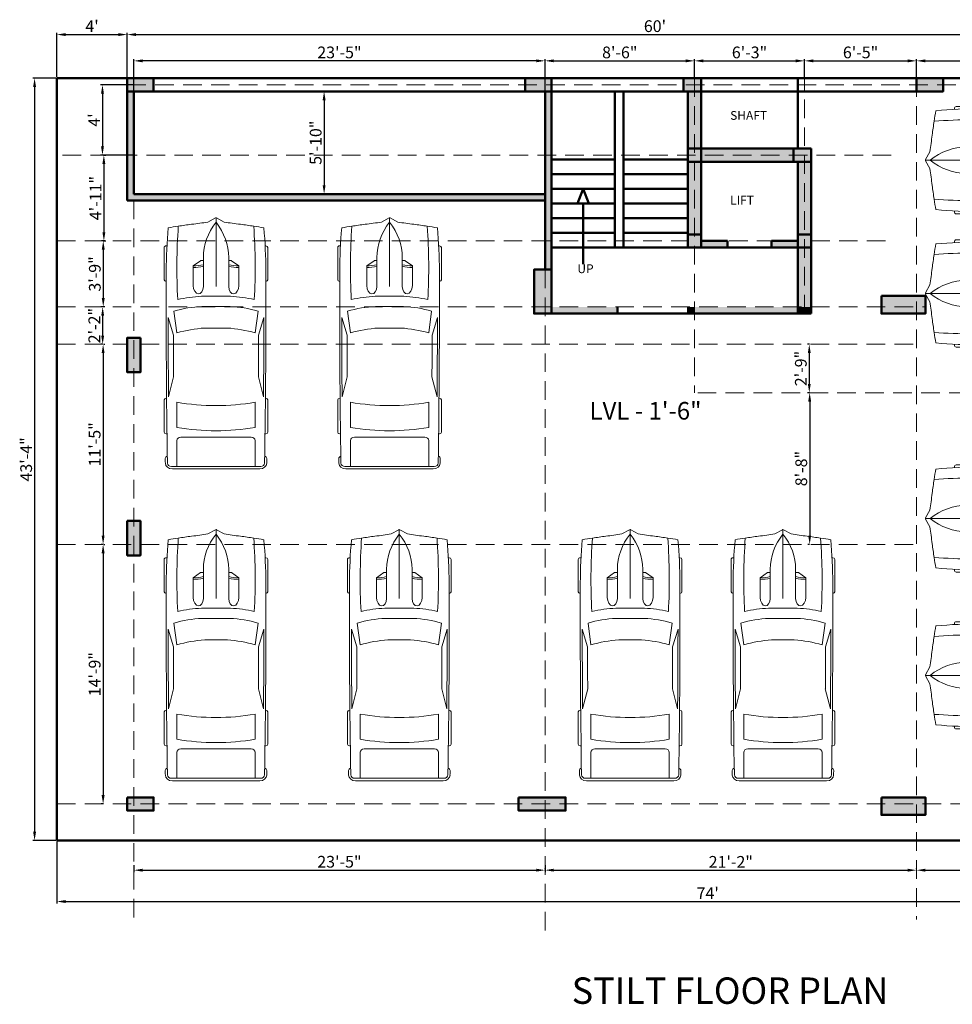
# Model space of a CAD drawing. Units: millimetres. Extents: x 1706 to 5913, y 156 to 1716.
# Tile 6 of 26: x 1714 to 2350, y 1031 to 1702. Entities that reach past the tile are written whole.
import ezdxf

# ---------------------------------------------------------------- set-up
doc = ezdxf.new("R2010")
doc.units = ezdxf.units.MM
doc.linetypes.add('DASHED', pattern=[19.05, 12.7, -6.35])
for name, color, linetype, lineweight in [('A-ANNO-DIMS', 2, 'Continuous', 18), ('A-ANNO-SYMB', 3, 'Continuous', 18), ('A-ANNO-TEXT', 7, 'Continuous', 18), ('A-AREA-IDEN', 3, 'Continuous', 18), ('A-COLS', 20, 'Continuous', 50), ('A-EQPM', 8, 'Continuous', 18), ('A-FLOR-OVHD', 9, 'DASHED', 18), ('A-WALL', 7, 'Continuous', 50), ('A-WALL-PATT', 252, 'Continuous', 13)]:
    doc.layers.add(name, color=color, linetype=linetype, lineweight=lineweight)
doc.styles.get("Standard").update_dxf_attribs({"font": 'arial.ttf'})
doc.dimstyles.new('ISO-25', dxfattribs={"dimtxt": 8, "dimasz": 6, "dimexe": 1.25, "dimexo": 0.625, "dimtad": 1, "dimdec": 0, "dimlunit": 3, "dimtxsty": 'Standard', "dimcen": 2.5, "dimadec": 0, "dimazin": 0, "dimtfac": 1, "dimtdec": 0, "dimtmove": 0, "dimatfit": 3, "dimfxl": 1, "dimarcsym": 0})

# ---------------------------------------------------------------- blocks, each defined once
blk = doc.blocks.new('*D81')
at = {"layer": 'A-ANNO-DIMS', "color": 0, "lineweight": -2, "transparency": 16777216}
for p, q in [((1771.16, 1609.78), (1772.72, 1609.78)), ((1771.47, 1603.78), (1771.47, 1557.28)), ((1771.16, 1551.28), (1772.72, 1551.28))]:
    blk.add_line(p, q, dxfattribs=at)
at = {"layer": 'A-ANNO-DIMS', "color": 0, "transparency": 16777216}
for points in [[(1770.47, 1603.78), (1772.47, 1603.78), (1771.47, 1609.78)], [(1770.47, 1557.28), (1772.47, 1557.28), (1771.47, 1551.28)]]:
    blk.add_solid(points, dxfattribs=at)
at = {"layer": 'Defpoints', "color": 0, "transparency": 16777216}
for p in [(1770.53, 1609.78), (1770.53, 1551.28), (1771.47, 1551.28)]:
    blk.add_point(p, dxfattribs=at)
at = {"layer": 'A-ANNO-DIMS', "color": 0, "transparency": 16777216, "insert": (1766.83, 1580.53), "char_height": 8, "attachment_point": 5, "rotation": 90}
blk.add_mtext('4\'-11"', dxfattribs=at)
blk = doc.blocks.new('*D82')
at = {"layer": 'A-ANNO-DIMS', "color": 0, "lineweight": -2, "transparency": 16777216}
for p, q in [((1772.1, 1551.28), (1769.8, 1551.28)), ((1771.05, 1545.28), (1771.05, 1512.28)), ((1772.1, 1506.28), (1769.8, 1506.28))]:
    blk.add_line(p, q, dxfattribs=at)
at = {"layer": 'A-ANNO-DIMS', "color": 0, "transparency": 16777216}
for points in [[(1770.05, 1545.28), (1772.05, 1545.28), (1771.05, 1551.28)], [(1770.05, 1512.28), (1772.05, 1512.28), (1771.05, 1506.28)]]:
    blk.add_solid(points, dxfattribs=at)
at = {"layer": 'Defpoints', "color": 0, "transparency": 16777216}
for p in [(1772.72, 1551.28), (1771.05, 1506.28), (1772.72, 1506.28)]:
    blk.add_point(p, dxfattribs=at)
at = {"layer": 'A-ANNO-DIMS', "color": 0, "transparency": 16777216, "insert": (1766.34, 1528.78), "char_height": 8, "attachment_point": 5, "rotation": 90}
blk.add_mtext('3\'-9"', dxfattribs=at)
blk = doc.blocks.new('*U10')
for p, q in [((21.1, 37.41), (21.1, 36.83)), ((46.55, 38.89), (22.35, 38.89)), ((47.8, 37.39), (47.8, 37.41)), ((87.99, 31.87), (74.76, 35.92)), ((135.45, 37.07), (135.45, 37.41)), ((136.7, 38.89), (160.9, 38.89)), ((162.15, 37.41), (162.15, 36.77)), ((70.03, 31.54), (86.41, 29.35)), ((134.31, 35.6), (119.29, 31.78)), ((138.42, 29.35), (157.25, 29.35)), ((186.47, 29.35), (167.01, 29.35)), ((186.47, -33.5), (186.47, 33.5)), ((188.4, -32.76), (188.4, 32.76)), ((164.52, 26.39), (164.52, -26.39)), ((32.27, 11.63), (36.13, 17.17)), ((36.13, 17.17), (50.94, 17.17)), ((29.77, 9.51), (51.68, 9.51)), ((32.12, 9.51), (32.12, 11.15)), ((58.92, -10.77), (58.92, 10.77)), ((66.55, -10.53), (66.55, 10.53)), ((82.74, 8.5), (82.74, -8.5)), ((186.47, -10.53), (186.47, 10.53)), ((3.27, 6.13), (0.1, 0.41)), ((0, 0), (51.68, 0)), ((0.1, -0.41), (3.27, -6.13)), ((29.77, -9.51), (51.68, -9.51)), ((32.12, -9.51), (32.12, -11.15)), ((32.27, -11.63), (36.13, -17.17)), ((36.13, -17.17), (50.94, -17.17)), ((86.41, -29.35), (70.03, -31.54)), ((87.99, -31.87), (74.76, -35.92)), ((134.31, -35.6), (119.29, -31.78)), ((157.25, -29.35), (138.42, -29.35)), ((167.01, -29.35), (186.47, -29.35)), ((21.1, -37.41), (21.1, -36.83)), ((46.55, -38.89), (22.35, -38.89)), ((47.8, -37.39), (47.8, -37.41)), ((135.45, -37.07), (135.45, -37.41)), ((136.7, -38.89), (160.9, -38.89)), ((162.15, -37.41), (162.15, -36.77))]:
    blk.add_line(p, q)
for centre, major_axis, ratio, start_param, end_param in [((266.03, -27.52), (0, 313.31), 0.842304, 1.367076, 1.39176), ((41.19, -490.86), (0, 528.23), 0.842304, 0.00281, 0.075598), ((22.35, 37.41), (0, -1.48), 0.842304, 3.141593, 4.712389), ((64.48, -10555.62), (0, 10593.03), 0.842304, -0.013397, 0.002797), ((46.55, 37.41), (0, 1.48), 0.842304, -1.570796, 0), ((64.48, -10555.62), (0, -10591.55), 0.842304, 3.133765, 3.140441), ((136.7, 37.41), (0, -1.48), 0.842304, 3.141593, 4.712389), ((160.9, 37.41), (0, 1.48), 0.842304, -1.570796, 0), ((180.63, 35.84), (0, 2.22), 0.842304, -0.013017, 1.249894), ((64.48, -10556.36), (0, 10595.31), 0.842304, -0.013397, -0.013017), ((183.98, 33.5), (0, -2.96), 0.842304, 1.570796, 3.128196), ((183.98, 32.76), (0, -5.25), 0.842304, 1.570796, 3.128196), ((37.47, -593.96), (0, -623.33), 0.842304, 3.096046, 3.200911), ((134.4, 5.39), (0, -89.78), 0.842304, 4.449482, 4.652344), ((135.29, 5.39), (0, 81.77), 0.842304, 1.245306, 1.50788), ((149.6, 2.8), (0, -79.58), 0.842304, 4.372215, 4.640744), ((95.79, -3666.35), (0, -3698.24), 0.842304, 3.134049, 3.144098), ((17.08, 0), (0, 147.02), 0.842304, 4.511394, 4.913384), ((35.91, 0), (0, 147.02), 0.842304, 4.511394, 4.913384), ((167.01, 26.39), (0, 2.96), 0.842304, 0, 1.570796), ((259.18, -27.52), (0, -305.3), 0.842304, 4.528606, 4.561838), ((-204.49, 52.4), (0, -250.96), 0.842304, 1.385369, 1.434372), ((13.04, 17.01), (0, 27.42), 0.842304, 4.435146, 4.718221), ((14.2, 17.01), (0, 27.42), 0.842304, 4.435146, 4.718221), ((50.79, 13.34), (6.34, -0.36), 0.603834, -1.395552, 1.581315), ((29.77, -46.66), (0, 56.17), 0.842304, 0, 0.590319), ((32.75, 11.15), (0, 0.74), 0.842304, 0.879714, 1.570796), ((0.62, 0), (0, -0.74), 0.842304, 4.131459, 5.293319), ((-204.49, -52.4), (0, 250.96), 0.842304, -1.434372, -1.385369), ((29.77, 46.66), (0, 56.17), 0.842304, 2.551274, 3.141593), ((32.75, -11.15), (0, -0.74), 0.842304, 4.712389, 5.403472), ((13.04, -17.01), (0, -27.42), 0.842304, 1.564964, 1.848039), ((14.2, -17.01), (0, -27.42), 0.842304, 1.564964, 1.848039), ((134.4, -5.39), (0, -89.78), 0.842304, -1.510751, -1.307889), ((135.29, -5.39), (0, -81.77), 0.842304, -1.50788, -1.245306), ((149.6, -2.8), (0, -79.58), 0.842304, -1.499151, -1.230623), ((259.18, 27.52), (0, 305.3), 0.842304, 1.721348, 1.754579), ((266.03, 27.52), (0, 313.31), 0.842304, 1.749832, 1.774517), ((37.47, 593.96), (0, -623.33), 0.842304, -0.059319, 0.045547), ((167.01, -26.39), (0, -2.96), 0.842304, 4.712389, 6.283185), ((64.48, 10555.62), (0, -10591.55), 0.842304, 0.001152, 0.007828), ((95.79, 3666.35), (0, -3698.24), 0.842304, -0.002505, 0.007544), ((183.98, -33.5), (0, 2.96), 0.842304, 3.15499, 4.712389), ((183.98, -32.76), (0, -5.25), 0.842304, 0.013397, 1.570796), ((41.19, 490.86), (0, -528.23), 0.842304, -0.075598, -0.00281), ((22.35, -37.41), (0, 1.48), 0.842304, 1.570796, 3.141593), ((64.48, 10555.62), (0, 10593.03), 0.842304, 3.138796, 3.15499), ((46.55, -37.41), (0, -1.48), 0.842304, 0, 1.570796), ((136.7, -37.41), (0, -1.48), 0.842304, -1.570796, 0), ((160.9, -37.41), (0, 1.48), 0.842304, 3.141593, 4.712389), ((180.63, -35.84), (0, -2.22), 0.842304, -1.249894, 0.013017), ((64.48, 10556.36), (0, 10595.31), 0.842304, 3.15461, 3.15499)]:
    blk.add_ellipse(centre, major_axis=major_axis, ratio=ratio, start_param=start_param, end_param=end_param)
at = {"extrusion": (0, 0, -1)}
blk.add_ellipse((50.79, -13.34), major_axis=(6.34, 0.36), ratio=0.603834, start_param=-1.395552, end_param=1.581315, dxfattribs=at)
blk = doc.blocks.new('*D85')
at = {"layer": 'A-ANNO-DIMS', "color": 0, "lineweight": -2, "transparency": 16777216}
for p, q in [((1770.33, 1506.28), (1769.39, 1506.28)), ((1770.64, 1500.28), (1770.64, 1486.78)), ((1770.33, 1480.78), (1769.39, 1480.78))]:
    blk.add_line(p, q, dxfattribs=at)
at = {"layer": 'A-ANNO-DIMS', "color": 0, "transparency": 16777216}
for points in [[(1769.64, 1500.28), (1771.64, 1500.28), (1770.64, 1506.28)], [(1769.64, 1486.78), (1771.64, 1486.78), (1770.64, 1480.78)]]:
    blk.add_solid(points, dxfattribs=at)
at = {"layer": 'Defpoints', "color": 0, "transparency": 16777216}
for p in [(1770.95, 1506.28), (1770.64, 1480.78), (1770.95, 1480.78)]:
    blk.add_point(p, dxfattribs=at)
at = {"layer": 'A-ANNO-DIMS', "color": 0, "transparency": 16777216, "insert": (1766, 1493.53), "char_height": 8, "attachment_point": 5, "rotation": 90}
blk.add_mtext('2\'-2"', dxfattribs=at)
blk = doc.blocks.new('*D86')
at = {"layer": 'A-ANNO-DIMS', "color": 0, "lineweight": -2, "transparency": 16777216}
for p, q in [((1771.58, 1480.78), (1772.2, 1480.78)), ((1770.95, 1474.78), (1770.95, 1350.28)), ((1771.58, 1344.28), (1772.2, 1344.28))]:
    blk.add_line(p, q, dxfattribs=at)
at = {"layer": 'A-ANNO-DIMS', "color": 0, "transparency": 16777216}
for points in [[(1769.95, 1474.78), (1771.95, 1474.78), (1770.95, 1480.78)], [(1769.95, 1350.28), (1771.95, 1350.28), (1770.95, 1344.28)]]:
    blk.add_solid(points, dxfattribs=at)
at = {"layer": 'Defpoints', "color": 0, "transparency": 16777216}
for p in [(1770.95, 1480.78), (1770.95, 1344.28), (1770.95, 1344.28)]:
    blk.add_point(p, dxfattribs=at)
at = {"layer": 'A-ANNO-DIMS', "color": 0, "transparency": 16777216, "insert": (1766.24, 1412.53), "char_height": 8, "attachment_point": 5, "rotation": 90}
blk.add_mtext('11\'-5"', dxfattribs=at)
blk = doc.blocks.new('*D87')
at = {"layer": 'A-ANNO-DIMS', "color": 0, "lineweight": -2, "transparency": 16777216}
for p, q in [((1771.26, 1344.28), (1769.7, 1344.28)), ((1770.95, 1338.28), (1770.95, 1173.28)), ((1771.26, 1167.28), (1769.7, 1167.28))]:
    blk.add_line(p, q, dxfattribs=at)
at = {"layer": 'A-ANNO-DIMS', "color": 0, "transparency": 16777216}
for points in [[(1769.95, 1338.28), (1771.95, 1338.28), (1770.95, 1344.28)], [(1769.95, 1173.28), (1771.95, 1173.28), (1770.95, 1167.28)]]:
    blk.add_solid(points, dxfattribs=at)
at = {"layer": 'Defpoints', "color": 0, "transparency": 16777216}
for p in [(1771.89, 1344.28), (1770.95, 1167.28), (1771.89, 1167.28)]:
    blk.add_point(p, dxfattribs=at)
at = {"layer": 'A-ANNO-DIMS', "color": 0, "transparency": 16777216, "insert": (1766.24, 1255.78), "char_height": 8, "attachment_point": 5, "rotation": 90}
blk.add_mtext('14\'-9"', dxfattribs=at)
blk = doc.blocks.new('*D88')
at = {"layer": 'A-ANNO-DIMS', "color": 0, "lineweight": -2, "transparency": 16777216}
for p, q in [((1791.9, 1125.52), (1791.9, 1120.84)), ((1797.9, 1122.09), (2066.4, 1122.09)), ((2072.4, 1125.52), (2072.4, 1120.84))]:
    blk.add_line(p, q, dxfattribs=at)
at = {"layer": 'A-ANNO-DIMS', "color": 0, "transparency": 16777216}
for points in [[(1797.9, 1123.09), (1797.9, 1121.09), (1791.9, 1122.09)], [(2066.4, 1123.09), (2066.4, 1121.09), (2072.4, 1122.09)]]:
    blk.add_solid(points, dxfattribs=at)
at = {"layer": 'Defpoints', "color": 0, "transparency": 16777216}
for p in [(1791.9, 1126.15), (2072.4, 1126.15), (2072.4, 1122.09)]:
    blk.add_point(p, dxfattribs=at)
at = {"layer": 'A-ANNO-DIMS', "color": 0, "transparency": 16777216, "insert": (1932.15, 1126.8), "char_height": 8, "attachment_point": 5}
blk.add_mtext('23\'-5"', dxfattribs=at)
blk = doc.blocks.new('*D89')
at = {"layer": 'A-ANNO-DIMS', "color": 0, "lineweight": -2, "transparency": 16777216}
for p, q in [((2072.4, 1122.72), (2072.4, 1123.34)), ((2078.4, 1122.09), (2319.9, 1122.09)), ((2325.9, 1122.72), (2325.9, 1123.34))]:
    blk.add_line(p, q, dxfattribs=at)
at = {"layer": 'A-ANNO-DIMS', "color": 0, "transparency": 16777216}
for points in [[(2078.4, 1123.09), (2078.4, 1121.09), (2072.4, 1122.09)], [(2319.9, 1123.09), (2319.9, 1121.09), (2325.9, 1122.09)]]:
    blk.add_solid(points, dxfattribs=at)
at = {"layer": 'Defpoints', "color": 0, "transparency": 16777216}
for p in [(2072.4, 1122.09), (2325.9, 1122.09), (2325.9, 1122.09)]:
    blk.add_point(p, dxfattribs=at)
at = {"layer": 'A-ANNO-DIMS', "color": 0, "transparency": 16777216, "insert": (2199.15, 1126.73), "char_height": 8, "attachment_point": 5}
blk.add_mtext('21\'-2"', dxfattribs=at)
blk = doc.blocks.new('*D90')
at = {"layer": 'A-ANNO-DIMS', "color": 0, "lineweight": -2, "transparency": 16777216}
for p, q in [((2325.9, 1122.72), (2325.9, 1123.34)), ((2331.9, 1122.09), (2501.4, 1122.09)), ((2507.4, 1122.72), (2507.4, 1123.34))]:
    blk.add_line(p, q, dxfattribs=at)
at = {"layer": 'A-ANNO-DIMS', "color": 0, "transparency": 16777216}
for points in [[(2331.9, 1123.09), (2331.9, 1121.09), (2325.9, 1122.09)], [(2501.4, 1123.09), (2501.4, 1121.09), (2507.4, 1122.09)]]:
    blk.add_solid(points, dxfattribs=at)
at = {"layer": 'Defpoints', "color": 0, "transparency": 16777216}
for p in [(2325.9, 1122.09), (2507.4, 1122.09), (2507.4, 1122.09)]:
    blk.add_point(p, dxfattribs=at)
at = {"layer": 'A-ANNO-DIMS', "color": 0, "transparency": 16777216, "insert": (2416.65, 1126.8), "char_height": 8, "attachment_point": 5}
blk.add_mtext('15\'-2"', dxfattribs=at)
blk = doc.blocks.new('*D92')
at = {"layer": 'A-ANNO-DIMS', "color": 0, "lineweight": -2, "transparency": 16777216}
for p, q in [((1791.9, 1653.9), (1791.9, 1675.38)), ((2066.4, 1674.13), (1797.9, 1674.13)), ((2072.4, 1653.9), (2072.4, 1675.38))]:
    blk.add_line(p, q, dxfattribs=at)
at = {"layer": 'A-ANNO-DIMS', "color": 0, "transparency": 16777216}
for points in [[(1797.9, 1675.13), (1797.9, 1673.13), (1791.9, 1674.13)], [(2066.4, 1675.13), (2066.4, 1673.13), (2072.4, 1674.13)]]:
    blk.add_solid(points, dxfattribs=at)
at = {"layer": 'Defpoints', "color": 0, "transparency": 16777216}
for p in [(1791.9, 1674.13), (1791.9, 1653.28), (2072.4, 1653.28)]:
    blk.add_point(p, dxfattribs=at)
at = {"layer": 'A-ANNO-DIMS', "color": 0, "transparency": 16777216, "insert": (1932.15, 1678.84), "char_height": 8, "attachment_point": 5}
blk.add_mtext('23\'-5"', dxfattribs=at)
blk = doc.blocks.new('*D93')
at = {"layer": 'A-ANNO-DIMS', "color": 0, "lineweight": -2, "transparency": 16777216}
for p, q in [((2072.4, 1662.9), (2072.4, 1675.38)), ((2078.4, 1674.13), (2168.4, 1674.13)), ((2174.4, 1662.9), (2174.4, 1675.38))]:
    blk.add_line(p, q, dxfattribs=at)
at = {"layer": 'A-ANNO-DIMS', "color": 0, "transparency": 16777216}
for points in [[(2078.4, 1675.13), (2078.4, 1673.13), (2072.4, 1674.13)], [(2168.4, 1675.13), (2168.4, 1673.13), (2174.4, 1674.13)]]:
    blk.add_solid(points, dxfattribs=at)
at = {"layer": 'Defpoints', "color": 0, "transparency": 16777216}
for p in [(2174.4, 1674.13), (2072.4, 1662.28), (2174.4, 1662.28)]:
    blk.add_point(p, dxfattribs=at)
at = {"layer": 'A-ANNO-DIMS', "color": 0, "transparency": 16777216, "insert": (2123.4, 1678.84), "char_height": 8, "attachment_point": 5}
blk.add_mtext('8\'-6"', dxfattribs=at)
blk = doc.blocks.new('*D94')
at = {"layer": 'A-ANNO-DIMS', "color": 0, "lineweight": -2, "transparency": 16777216}
for p, q in [((2174.4, 1662.9), (2174.4, 1675.38)), ((2180.4, 1674.13), (2243.4, 1674.13)), ((2249.4, 1662.9), (2249.4, 1675.38))]:
    blk.add_line(p, q, dxfattribs=at)
at = {"layer": 'A-ANNO-DIMS', "color": 0, "transparency": 16777216}
for points in [[(2180.4, 1675.13), (2180.4, 1673.13), (2174.4, 1674.13)], [(2243.4, 1675.13), (2243.4, 1673.13), (2249.4, 1674.13)]]:
    blk.add_solid(points, dxfattribs=at)
at = {"layer": 'Defpoints', "color": 0, "transparency": 16777216}
for p in [(2249.4, 1674.13), (2174.4, 1662.28), (2249.4, 1662.28)]:
    blk.add_point(p, dxfattribs=at)
at = {"layer": 'A-ANNO-DIMS', "color": 0, "transparency": 16777216, "insert": (2211.9, 1678.84), "char_height": 8, "attachment_point": 5}
blk.add_mtext('6\'-3"', dxfattribs=at)
blk = doc.blocks.new('*D95')
at = {"layer": 'A-ANNO-DIMS', "color": 0, "lineweight": -2, "transparency": 16777216}
for p, q in [((2249.4, 1662.9), (2249.4, 1675.38)), ((2255.4, 1674.13), (2319.9, 1674.13)), ((2325.9, 1662.9), (2325.9, 1675.38))]:
    blk.add_line(p, q, dxfattribs=at)
at = {"layer": 'A-ANNO-DIMS', "color": 0, "transparency": 16777216}
for points in [[(2255.4, 1675.13), (2255.4, 1673.13), (2249.4, 1674.13)], [(2319.9, 1675.13), (2319.9, 1673.13), (2325.9, 1674.13)]]:
    blk.add_solid(points, dxfattribs=at)
at = {"layer": 'Defpoints', "color": 0, "transparency": 16777216}
for p in [(2325.9, 1674.13), (2249.4, 1662.28), (2325.9, 1662.28)]:
    blk.add_point(p, dxfattribs=at)
at = {"layer": 'A-ANNO-DIMS', "color": 0, "transparency": 16777216, "insert": (2287.65, 1678.84), "char_height": 8, "attachment_point": 5}
blk.add_mtext('6\'-5"', dxfattribs=at)
blk = doc.blocks.new('*D96')
at = {"layer": 'A-ANNO-DIMS', "color": 0, "lineweight": -2, "transparency": 16777216}
for p, q in [((2325.9, 1662.9), (2325.9, 1675.38)), ((2331.9, 1674.13), (2501.4, 1674.13)), ((2507.4, 1662.9), (2507.4, 1675.38))]:
    blk.add_line(p, q, dxfattribs=at)
at = {"layer": 'A-ANNO-DIMS', "color": 0, "transparency": 16777216}
for points in [[(2331.9, 1675.13), (2331.9, 1673.13), (2325.9, 1674.13)], [(2501.4, 1675.13), (2501.4, 1673.13), (2507.4, 1674.13)]]:
    blk.add_solid(points, dxfattribs=at)
at = {"layer": 'Defpoints', "color": 0, "transparency": 16777216}
for p in [(2507.4, 1674.13), (2325.9, 1662.28), (2507.4, 1662.28)]:
    blk.add_point(p, dxfattribs=at)
at = {"layer": 'A-ANNO-DIMS', "color": 0, "transparency": 16777216, "insert": (2416.65, 1678.84), "char_height": 8, "attachment_point": 5}
blk.add_mtext('15\'-2"', dxfattribs=at)
blk = doc.blocks.new('*D97')
at = {"layer": 'A-ANNO-DIMS', "color": 0, "lineweight": -2, "transparency": 16777216}
for p, q in [((2252.8, 1480.78), (2251.41, 1480.78)), ((2252.66, 1474.78), (2252.66, 1453.78)), ((2252.8, 1447.78), (2251.41, 1447.78))]:
    blk.add_line(p, q, dxfattribs=at)
at = {"layer": 'A-ANNO-DIMS', "color": 0, "transparency": 16777216}
for points in [[(2251.66, 1474.78), (2253.66, 1474.78), (2252.66, 1480.78)], [(2251.66, 1453.78), (2253.66, 1453.78), (2252.66, 1447.78)]]:
    blk.add_solid(points, dxfattribs=at)
at = {"layer": 'Defpoints', "color": 0, "transparency": 16777216}
for p in [(2253.42, 1480.78), (2252.66, 1447.78), (2253.42, 1447.78)]:
    blk.add_point(p, dxfattribs=at)
at = {"layer": 'A-ANNO-DIMS', "color": 0, "transparency": 16777216, "insert": (2247.95, 1464.28), "char_height": 8, "attachment_point": 5, "rotation": 90}
blk.add_mtext('2\'-9"', dxfattribs=at)
blk = doc.blocks.new('*D98')
at = {"layer": 'A-ANNO-DIMS', "color": 0, "lineweight": -2, "transparency": 16777216}
for p, q in [((2252.8, 1447.78), (2251.69, 1447.78)), ((2252.94, 1441.78), (2252.94, 1350.28)), ((2252.8, 1344.28), (2251.69, 1344.28))]:
    blk.add_line(p, q, dxfattribs=at)
at = {"layer": 'A-ANNO-DIMS', "color": 0, "transparency": 16777216}
for points in [[(2251.94, 1441.78), (2253.94, 1441.78), (2252.94, 1447.78)], [(2251.94, 1350.28), (2253.94, 1350.28), (2252.94, 1344.28)]]:
    blk.add_solid(points, dxfattribs=at)
at = {"layer": 'Defpoints', "color": 0, "transparency": 16777216}
for p in [(2253.42, 1447.78), (2252.94, 1344.28), (2253.42, 1344.28)]:
    blk.add_point(p, dxfattribs=at)
at = {"layer": 'A-ANNO-DIMS', "color": 0, "transparency": 16777216, "insert": (2248.23, 1396.03), "char_height": 8, "attachment_point": 5, "rotation": 90}
blk.add_mtext('8\'-8"', dxfattribs=at)
blk = doc.blocks.new('*D99')
at = {"layer": 'A-ANNO-DIMS', "color": 0, "lineweight": -2, "transparency": 16777216}
for p, q in [((1739.4, 1141.65), (1739.4, 1099.48)), ((2627.4, 1141.65), (2627.4, 1099.48)), ((1745.4, 1100.73), (2621.4, 1100.73))]:
    blk.add_line(p, q, dxfattribs=at)
at = {"layer": 'A-ANNO-DIMS', "color": 0, "transparency": 16777216}
for points in [[(1745.4, 1101.73), (1745.4, 1099.73), (1739.4, 1100.73)], [(2621.4, 1101.73), (2621.4, 1099.73), (2627.4, 1100.73)]]:
    blk.add_solid(points, dxfattribs=at)
at = {"layer": 'Defpoints', "color": 0, "transparency": 16777216}
for p in [(1739.4, 1142.28), (2627.4, 1142.28), (2627.4, 1100.73)]:
    blk.add_point(p, dxfattribs=at)
at = {"layer": 'A-ANNO-DIMS', "color": 0, "transparency": 16777216, "insert": (2183.4, 1105.35), "char_height": 8, "attachment_point": 5}
blk.add_mtext("74'", dxfattribs=at)
blk = doc.blocks.new('*D100')
at = {"layer": 'A-ANNO-DIMS', "color": 0, "lineweight": -2, "transparency": 16777216}
for p, q in [((1787.4, 1662.9), (1787.4, 1693.3)), ((2507.4, 1662.9), (2507.4, 1693.3)), ((1793.4, 1692.05), (2501.4, 1692.05))]:
    blk.add_line(p, q, dxfattribs=at)
at = {"layer": 'A-ANNO-DIMS', "color": 0, "transparency": 16777216}
for points in [[(1793.4, 1693.05), (1793.4, 1691.05), (1787.4, 1692.05)], [(2501.4, 1693.05), (2501.4, 1691.05), (2507.4, 1692.05)]]:
    blk.add_solid(points, dxfattribs=at)
at = {"layer": 'Defpoints', "color": 0, "transparency": 16777216}
for p in [(2507.4, 1692.05), (1787.4, 1662.28), (2507.4, 1662.28)]:
    blk.add_point(p, dxfattribs=at)
at = {"layer": 'A-ANNO-DIMS', "color": 0, "transparency": 16777216, "insert": (2147.4, 1696.76), "char_height": 8, "attachment_point": 5}
blk.add_mtext("60'", dxfattribs=at)
blk = doc.blocks.new('*D101')
at = {"layer": 'A-ANNO-DIMS', "color": 0, "lineweight": -2, "transparency": 16777216}
for p, q in [((1739.4, 1662.9), (1739.4, 1693.3)), ((1787.4, 1662.9), (1787.4, 1693.3)), ((1745.4, 1692.05), (1781.4, 1692.05))]:
    blk.add_line(p, q, dxfattribs=at)
at = {"layer": 'A-ANNO-DIMS', "color": 0, "transparency": 16777216}
for points in [[(1745.4, 1693.05), (1745.4, 1691.05), (1739.4, 1692.05)], [(1781.4, 1693.05), (1781.4, 1691.05), (1787.4, 1692.05)]]:
    blk.add_solid(points, dxfattribs=at)
at = {"layer": 'Defpoints', "color": 0, "transparency": 16777216}
for p in [(1787.4, 1692.05), (1739.4, 1662.28), (1787.4, 1662.28)]:
    blk.add_point(p, dxfattribs=at)
at = {"layer": 'A-ANNO-DIMS', "color": 0, "transparency": 16777216, "insert": (1763.4, 1696.67), "char_height": 8, "attachment_point": 5}
blk.add_mtext("4'", dxfattribs=at)
blk = doc.blocks.new('*D102')
at = {"layer": 'A-ANNO-DIMS', "color": 0, "lineweight": -2, "transparency": 16777216}
for p, q in [((1922.33, 1653.28), (1922.96, 1653.28)), ((1921.71, 1647.28), (1921.71, 1589.28)), ((1922.33, 1583.28), (1922.96, 1583.28))]:
    blk.add_line(p, q, dxfattribs=at)
at = {"layer": 'A-ANNO-DIMS', "color": 0, "transparency": 16777216}
for points in [[(1920.71, 1647.28), (1922.71, 1647.28), (1921.71, 1653.28)], [(1920.71, 1589.28), (1922.71, 1589.28), (1921.71, 1583.28)]]:
    blk.add_solid(points, dxfattribs=at)
at = {"layer": 'Defpoints', "color": 0, "transparency": 16777216}
for p in [(1921.71, 1653.28), (1921.71, 1583.28), (1921.71, 1583.28)]:
    blk.add_point(p, dxfattribs=at)
at = {"layer": 'A-ANNO-DIMS', "color": 0, "transparency": 16777216, "insert": (1917, 1618.28), "char_height": 8, "attachment_point": 5, "rotation": 90}
blk.add_mtext('5\'-10"', dxfattribs=at)
blk = doc.blocks.new('*D103')
at = {"layer": 'A-ANNO-DIMS', "color": 0, "lineweight": -2, "transparency": 16777216}
for p, q in [((1791.28, 1657.78), (1769.28, 1657.78)), ((1770.53, 1651.78), (1770.53, 1615.78)), ((1791.28, 1609.78), (1769.28, 1609.78))]:
    blk.add_line(p, q, dxfattribs=at)
at = {"layer": 'A-ANNO-DIMS', "color": 0, "transparency": 16777216}
for points in [[(1769.53, 1651.78), (1771.53, 1651.78), (1770.53, 1657.78)], [(1769.53, 1615.78), (1771.53, 1615.78), (1770.53, 1609.78)]]:
    blk.add_solid(points, dxfattribs=at)
at = {"layer": 'Defpoints', "color": 0, "transparency": 16777216}
for p in [(1791.9, 1657.78), (1770.53, 1609.78), (1791.9, 1609.78)]:
    blk.add_point(p, dxfattribs=at)
at = {"layer": 'A-ANNO-DIMS', "color": 0, "transparency": 16777216, "insert": (1765.91, 1633.78), "char_height": 8, "attachment_point": 5, "rotation": 90}
blk.add_mtext("4'", dxfattribs=at)
blk = doc.blocks.new('*D84')
at = {"layer": 'A-ANNO-DIMS', "color": 0, "lineweight": -2, "transparency": 16777216}
for p, q in [((1738.78, 1662.28), (1722.96, 1662.28)), ((1724.21, 1656.28), (1724.21, 1148.28)), ((1738.78, 1142.28), (1722.96, 1142.28))]:
    blk.add_line(p, q, dxfattribs=at)
at = {"layer": 'A-ANNO-DIMS', "color": 0, "transparency": 16777216}
for points in [[(1723.21, 1656.28), (1725.21, 1656.28), (1724.21, 1662.28)], [(1723.21, 1148.28), (1725.21, 1148.28), (1724.21, 1142.28)]]:
    blk.add_solid(points, dxfattribs=at)
at = {"layer": 'Defpoints', "color": 0, "transparency": 16777216}
for p in [(1739.4, 1662.28), (1724.21, 1142.28), (1739.4, 1142.28)]:
    blk.add_point(p, dxfattribs=at)
at = {"layer": 'A-ANNO-DIMS', "color": 0, "transparency": 16777216, "insert": (1719.5, 1402.28), "char_height": 8, "attachment_point": 5, "rotation": 90}
blk.add_mtext('43\'-4"', dxfattribs=at)

msp = doc.modelspace()

# ---------------------------------------------------------------- hatches: boundary and pattern name
at = {"layer": 'A-COLS'}
h = msp.add_hatch(color=256, dxfattribs=at)
h.dxf.hatch_style = 1
h.paths.add_polyline_path([(1805.4, 1662.28), (1787.4, 1662.28), (1787.4, 1653.28), (1805.4, 1653.28)])
h = msp.add_hatch(color=256, dxfattribs=at)
h.dxf.hatch_style = 1
h.paths.add_polyline_path([(2076.9, 1662.28), (2058.9, 1662.28), (2058.9, 1653.28), (2076.9, 1653.28)])
h = msp.add_hatch(color=256, dxfattribs=at)
h.dxf.hatch_style = 1
h.paths.add_polyline_path([(2178.9, 1662.28), (2166.9, 1662.28), (2166.9, 1653.28), (2178.9, 1653.28)])
h = msp.add_hatch(color=256, dxfattribs=at)
h.dxf.hatch_style = 1
h.paths.add_polyline_path([(2343.9, 1662.28), (2325.9, 1662.28), (2325.9, 1653.28), (2343.9, 1653.28)])
h = msp.add_hatch(color=256, dxfattribs=at)
h.dxf.hatch_style = 1
h.paths.add_polyline_path([(2178.9, 1614.28), (2169.9, 1614.28), (2169.9, 1605.28), (2178.9, 1605.28)])
h = msp.add_hatch(color=256, dxfattribs=at)
h.dxf.hatch_style = 1
h.paths.add_polyline_path([(2253.9, 1614.28), (2241.9, 1614.28), (2241.9, 1605.28), (2253.9, 1605.28)])
h = msp.add_hatch(color=256, dxfattribs=at)
h.dxf.hatch_style = 1
h.paths.add_polyline_path([(2178.9, 1555.78), (2169.9, 1555.78), (2169.9, 1546.78), (2178.9, 1546.78)])
h = msp.add_hatch(color=256, dxfattribs=at)
h.dxf.hatch_style = 1
h.paths.add_polyline_path([(2253.9, 1555.78), (2244.9, 1555.78), (2244.9, 1546.78), (2253.9, 1546.78)])
h = msp.add_hatch(color=256, dxfattribs=at)
h.dxf.hatch_style = 1
h.paths.add_polyline_path([(2076.9, 1531.78), (2064.9, 1531.78), (2064.9, 1501.78), (2076.9, 1501.78)])
h = msp.add_hatch(color=256, dxfattribs=at)
h.dxf.hatch_style = 1
h.paths.add_polyline_path([(2331.9, 1513.78), (2301.9, 1513.78), (2301.9, 1501.78), (2331.9, 1501.78)])
h = msp.add_hatch(color=256, dxfattribs=at)
h.dxf.hatch_style = 1
h.paths.add_polyline_path([(1796.4, 1485.28), (1787.4, 1485.28), (1787.4, 1461.78), (1796.4, 1461.78)])
h = msp.add_hatch(color=256, dxfattribs=at)
h.dxf.hatch_style = 1
h.paths.add_polyline_path([(1796.4, 1360.28), (1787.4, 1360.28), (1787.4, 1336.78), (1796.4, 1336.78)])
h = msp.add_hatch(color=256, dxfattribs=at)
h.dxf.hatch_style = 1
h.paths.add_polyline_path([(1805.4, 1171.78), (1787.4, 1171.78), (1787.4, 1162.78), (1805.4, 1162.78)])
h = msp.add_hatch(color=256, dxfattribs=at)
h.dxf.hatch_style = 1
h.paths.add_polyline_path([(2086.4, 1171.78), (2054.4, 1171.78), (2054.4, 1162.78), (2086.4, 1162.78)])
h = msp.add_hatch(color=256, dxfattribs=at)
h.dxf.hatch_style = 1
h.paths.add_polyline_path([(2331.9, 1171.78), (2301.9, 1171.78), (2301.9, 1159.78), (2331.9, 1159.78)])
at = {"layer": 'A-WALL-PATT'}
h = msp.add_hatch(color=256, dxfattribs=at)
h.dxf.hatch_style = 1
h.paths.add_polyline_path([(1791.9, 1653.28), (1787.4, 1653.28), (1787.4, 1609.78), (1791.9, 1609.78)])
h = msp.add_hatch(color=256, dxfattribs=at)
h.dxf.hatch_style = 1
h.paths.add_polyline_path([(2076.9, 1653.28), (2072.4, 1653.28), (2072.4, 1609.78), (2076.9, 1609.78)])
h = msp.add_hatch(color=256, dxfattribs=at)
h.dxf.hatch_style = 1
h.paths.add_polyline_path([(2174.4, 1653.28), (2169.9, 1653.28), (2169.9, 1614.28), (2174.4, 1614.28)])
h = msp.add_hatch(color=256, dxfattribs=at)
h.dxf.hatch_style = 1
h.paths.add_polyline_path([(2178.9, 1653.28), (2174.4, 1653.28), (2174.4, 1614.28), (2178.9, 1614.28)])
h = msp.add_hatch(color=256, dxfattribs=at)
h.dxf.hatch_style = 1
h.paths.add_polyline_path([(2241.9, 1614.28), (2178.9, 1614.28), (2178.9, 1609.78), (2241.9, 1609.78)])
h = msp.add_hatch(color=256, dxfattribs=at)
h.dxf.hatch_style = 1
h.paths.add_polyline_path([(1791.9, 1609.78), (1787.4, 1609.78), (1787.4, 1578.78), (2072.4, 1578.78), (2072.4, 1583.28), (1791.9, 1583.28)])
h = msp.add_hatch(color=256, dxfattribs=at)
h.dxf.hatch_style = 1
h.paths.add_polyline_path([(2076.9, 1609.78), (2072.4, 1609.78), (2072.4, 1551.28), (2076.9, 1551.28)])
h = msp.add_hatch(color=256, dxfattribs=at)
h.dxf.hatch_style = 1
h.paths.add_polyline_path([(2174.4, 1605.28), (2169.9, 1605.28), (2169.9, 1555.78), (2174.4, 1555.78)])
h = msp.add_hatch(color=256, dxfattribs=at)
h.dxf.hatch_style = 1
h.paths.add_polyline_path([(2178.9, 1605.28), (2174.4, 1605.28), (2174.4, 1555.78), (2178.9, 1555.78)])
h = msp.add_hatch(color=256, dxfattribs=at)
h.dxf.hatch_style = 1
h.paths.add_polyline_path([(2241.9, 1609.78), (2178.9, 1609.78), (2178.9, 1605.28), (2241.9, 1605.28)])
h = msp.add_hatch(color=256, dxfattribs=at)
h.dxf.hatch_style = 1
h.paths.add_polyline_path([(2249.4, 1605.28), (2244.9, 1605.28), (2244.9, 1555.78), (2249.4, 1555.78)])
h = msp.add_hatch(color=256, dxfattribs=at)
h.dxf.hatch_style = 1
h.paths.add_polyline_path([(2253.9, 1605.28), (2249.4, 1605.28), (2249.4, 1555.78), (2253.9, 1555.78)])
h = msp.add_hatch(color=256, dxfattribs=at)
h.dxf.hatch_style = 1
h.paths.add_polyline_path([(2076.9, 1551.28), (2072.4, 1551.28), (2072.4, 1531.78), (2076.9, 1531.78)])
h = msp.add_hatch(color=256, dxfattribs=at)
h.dxf.hatch_style = 1
h.paths.add_polyline_path([(2196.9, 1551.28), (2178.9, 1551.28), (2178.9, 1546.78), (2196.9, 1546.78)])
h = msp.add_hatch(color=256, dxfattribs=at)
h.dxf.hatch_style = 1
h.paths.add_polyline_path([(2244.9, 1551.28), (2226.9, 1551.28), (2226.9, 1546.78), (2244.9, 1546.78)])
h = msp.add_hatch(color=256, dxfattribs=at)
h.dxf.hatch_style = 1
h.paths.add_polyline_path([(2249.4, 1546.78), (2244.9, 1546.78), (2244.9, 1506.28), (2249.4, 1506.28)])
h = msp.add_hatch(color=256, dxfattribs=at)
h.dxf.hatch_style = 1
h.paths.add_polyline_path([(2253.9, 1546.78), (2249.4, 1546.78), (2249.4, 1506.28), (2253.9, 1506.28)])
h = msp.add_hatch(color=256, dxfattribs=at)
h.dxf.hatch_style = 1
h.paths.add_polyline_path([(2121.95, 1506.28), (2076.9, 1506.28), (2076.9, 1501.78), (2121.95, 1501.78)])
h = msp.add_hatch(color=256, dxfattribs=at)
h.dxf.hatch_style = 1
h.paths.add_polyline_path([(2174.4, 1506.28), (2169.95, 1506.28), (2169.95, 1501.78), (2174.4, 1501.78)])
h = msp.add_hatch(color=256, dxfattribs=at)
h.dxf.hatch_style = 1
h.paths.add_polyline_path([(2244.9, 1506.28), (2174.4, 1506.28), (2174.4, 1501.78), (2244.9, 1501.78)])
h = msp.add_hatch(color=256, dxfattribs=at)
h.dxf.hatch_style = 1
h.paths.add_polyline_path([(2249.4, 1506.28), (2244.9, 1506.28), (2244.9, 1501.78), (2249.4, 1501.78)])
h = msp.add_hatch(color=256, dxfattribs=at)
h.dxf.hatch_style = 1
h.paths.add_polyline_path([(2253.9, 1506.28), (2249.4, 1506.28), (2249.4, 1501.78), (2253.9, 1501.78)])

# ---------------------------------------------------------------- linework, layer by layer
at = {"layer": 'A-COLS'}
msp.add_lwpolyline([(1805.62, 1662.28), (1787.4, 1662.28), (1787.4, 1653.28), (1805.4, 1653.28), (1805.4, 1662.28)], dxfattribs=at)
for points in [[(2076.9, 1662.28), (2058.9, 1662.28), (2058.9, 1653.28), (2076.9, 1653.28)], [(2178.9, 1662.28), (2166.9, 1662.28), (2166.9, 1653.28), (2178.9, 1653.28)], [(2343.9, 1662.28), (2325.9, 1662.28), (2325.9, 1653.28), (2343.9, 1653.28)], [(2178.9, 1605.28), (2169.9, 1605.28), (2169.9, 1614.28), (2178.9, 1614.28)], [(2253.9, 1614.28), (2241.9, 1614.28), (2241.9, 1605.28), (2253.9, 1605.28)], [(2178.9, 1546.78), (2169.9, 1546.78), (2169.9, 1555.78), (2178.9, 1555.78)], [(2253.9, 1546.78), (2244.9, 1546.78), (2244.9, 1555.78), (2253.9, 1555.78)], [(2076.9, 1531.78), (2064.9, 1531.78), (2064.9, 1501.78), (2076.9, 1501.78)], [(2301.9, 1513.78), (2301.9, 1501.78), (2331.9, 1501.78), (2331.9, 1513.78)], [(1796.4, 1485.28), (1787.4, 1485.28), (1787.4, 1461.78), (1796.4, 1461.78)], [(1787.4, 1360.28), (1796.4, 1360.28), (1796.4, 1336.78), (1787.4, 1336.78)], [(1787.4, 1171.78), (1805.4, 1171.78), (1805.4, 1162.78), (1787.4, 1162.78)], [(2054.4, 1171.78), (2086.4, 1171.78), (2086.4, 1162.78), (2054.4, 1162.78)], [(2301.9, 1171.78), (2331.9, 1171.78), (2331.9, 1159.78), (2301.9, 1159.78)]]:
    msp.add_lwpolyline(points, close=True, dxfattribs=at)
at = {"layer": 'A-FLOR-OVHD'}
for p, q in [((2174.4, 1662.28), (2174.4, 1447.78)), ((2249.4, 1501.78), (2249.4, 1662.28)), ((2325.9, 1662.28), (2325.9, 1088.46)), ((1787.4, 1657.78), (2627.4, 1657.78)), ((2308.5, 1609.78), (1739.4, 1609.78)), ((1791.9, 1578.78), (1791.9, 1086.56)), ((1739.4, 1551.28), (2169.9, 1551.28)), ((2178.9, 1551.28), (2244.9, 1551.28)), ((2253.9, 1551.28), (2308.5, 1551.28)), ((2072.4, 1531.78), (2072.4, 1079.44)), ((1739.4, 1506.28), (2331.9, 1506.28)), ((1739.4, 1480.78), (1787.4, 1480.78)), ((1796.4, 1480.78), (2325.9, 1480.78)), ((2627.4, 1447.78), (2174.4, 1447.78)), ((1739.4, 1344.28), (2325.9, 1344.28)), ((1739.4, 1167.28), (2677.86, 1167.28))]:
    msp.add_line(p, q, dxfattribs=at)
at = {"layer": 'A-WALL'}
for p, q in [((1739.4, 1662.28), (2325.9, 1662.28)), ((1739.4, 1142.28), (1739.4, 1662.28)), ((1787.4, 1578.78), (1787.4, 1662.28)), ((1805.4, 1653.28), (1805.4, 1662.28)), ((2058.9, 1653.28), (2058.9, 1662.28)), ((2076.9, 1501.78), (2076.9, 1662.28)), ((2166.9, 1653.28), (2166.9, 1662.28)), ((2178.9, 1546.78), (2178.9, 1662.28)), ((2244.9, 1614.28), (2244.9, 1662.28)), ((2343.9, 1662.28), (2627.4, 1662.28)), ((1787.4, 1653.28), (2325.9, 1653.28)), ((1791.9, 1583.28), (1791.9, 1653.28)), ((2072.4, 1531.78), (2072.4, 1653.28)), ((2119.92, 1546.78), (2119.92, 1653.28)), ((2125.92, 1546.78), (2125.92, 1653.28)), ((2169.9, 1546.78), (2169.9, 1653.28)), ((2169.9, 1614.28), (2253.9, 1614.28)), ((2241.9, 1605.28), (2241.9, 1614.28)), ((2253.9, 1501.78), (2253.9, 1614.28)), ((2076.9, 1606.78), (2119.92, 1606.78)), ((2125.92, 1606.78), (2169.9, 1606.78)), ((2178.9, 1605.28), (2253.9, 1605.28)), ((2244.9, 1501.78), (2244.9, 1605.28)), ((2076.9, 1596.78), (2119.92, 1596.78)), ((2125.92, 1596.78), (2169.9, 1596.78)), ((2076.9, 1586.78), (2119.92, 1586.78)), ((2125.92, 1586.78), (2169.9, 1586.78)), ((1787.4, 1578.78), (2072.4, 1578.78)), ((1791.9, 1583.28), (2072.4, 1583.28)), ((2076.9, 1576.78), (2119.92, 1576.78)), ((2098.41, 1576.78), (2098.41, 1535.4)), ((2125.92, 1576.78), (2169.9, 1576.78)), ((2076.9, 1566.78), (2119.92, 1566.78)), ((2125.92, 1566.78), (2169.9, 1566.78)), ((2076.9, 1556.78), (2119.92, 1556.78)), ((2125.92, 1556.78), (2169.9, 1556.78)), ((2076.9, 1546.78), (2169.9, 1546.78)), ((2169.9, 1546.78), (2196.9, 1546.78)), ((2178.9, 1551.28), (2196.9, 1551.28)), ((2196.9, 1546.78), (2196.9, 1551.28)), ((2196.9, 1546.78), (2226.9, 1546.78)), ((2226.9, 1546.78), (2226.9, 1551.28)), ((2226.9, 1551.28), (2244.9, 1551.28)), ((2226.9, 1546.78), (2253.9, 1546.78)), ((2064.9, 1501.78), (2064.9, 1531.78)), ((2064.9, 1531.78), (2076.9, 1531.78)), ((2121.95, 1506.28), (2121.95, 1501.78)), ((2169.95, 1506.28), (2169.95, 1501.78)), ((2064.9, 1501.78), (2121.95, 1501.78)), ((2121.95, 1501.78), (2169.95, 1501.78)), ((2169.95, 1501.78), (2253.9, 1501.78)), ((2627.4, 1142.28), (1739.4, 1142.28))]:
    msp.add_line(p, q, dxfattribs=at)
msp.add_lwpolyline([(2098.41, 1586.78), (2102.36, 1576.78), (2094.46, 1576.78)], close=True, dxfattribs=at)

# ---------------------------------------------------------------- block references
at = {"layer": 'A-EQPM', "xscale": 0.9406440953584901, "yscale": 0.9406440953584901, "zscale": 0.9406440953584901}
for p in [(2331.86, 1606.37), (2331.86, 1515.48), (2331.86, 1361.99), (2331.86, 1254.99)]:
    msp.add_blockref('*U10', p, dxfattribs=at)
at = {"layer": 'A-EQPM', "xscale": 0.9095169601703508, "yscale": 0.9095169601703508, "zscale": 0.9095169601703508, "rotation": 270}
for p in [(1847.97, 1567.14), (1966.36, 1567.14), (1847.97, 1354.39), (1973.02, 1354.39), (2130.46, 1354.39), (2234.72, 1354.39)]:
    msp.add_blockref('*U10', p, dxfattribs=at)

# ---------------------------------------------------------------- texts
at = {"layer": 'A-ANNO-SYMB', "insert": (2102.77, 1441.43), "char_height": 12, "attachment_point": 1}
msp.add_mtext_dynamic_manual_height_columns('LVL - 1\'-6"', width=81.8676, gutter_width=12.5, heights=[0], dxfattribs=at)
at = {"layer": 'A-ANNO-TEXT', "attachment_point": 1}
for s, width, insert, char_height in [(' UP', 23.3743, (2092.64, 1535.34), 6), ('STILT FLOOR PLAN', 352.5721, (2090.6, 1048.93), 18)]:
    msp.add_mtext_dynamic_manual_height_columns(s, width=width, gutter_width=12.5, heights=[0], dxfattribs=dict(at, insert=insert, char_height=char_height))
at = {"layer": 'A-AREA-IDEN', "char_height": 6, "attachment_point": 1}
for s, insert in [('SHAFT', (2198.68, 1639.92)), ('LIFT', (2198.68, 1582.14))]:
    msp.add_mtext_dynamic_manual_height_columns(s, width=36.5395, gutter_width=12.5, heights=[0], dxfattribs=dict(at, insert=insert))

# ---------------------------------------------------------------- dimensions: what is measured, and where the dimension line sits
at = {"layer": 'A-ANNO-DIMS'}
for base, p1, p2, picture, middle in [((1787.4, 1692.05), (1739.4, 1662.28), (1787.4, 1662.28), '*D101', (1763.4, 1696.67)), ((2507.4, 1692.05), (1787.4, 1662.28), (2507.4, 1662.28), '*D100', (2147.4, 1696.76)), ((1791.9015753, 1674.12925326), (2072.4015753, 1653.27547118), (1791.9015753, 1653.27547118), '*D92', (1932.1515753, 1678.84156567)), ((2174.4, 1674.13), (2072.4, 1662.28), (2174.4, 1662.28), '*D93', (2123.4, 1678.84)), ((2249.4, 1674.13), (2174.4, 1662.28), (2249.4, 1662.28), '*D94', (2211.9, 1678.84)), ((2325.9015753, 1674.12925326), (2249.4015753, 1662.27547118), (2325.9015753, 1662.27547118), '*D95', (2287.6515753, 1678.83883716)), ((2507.4015753, 1674.12925326), (2325.9015753, 1662.27547118), (2507.4015753, 1662.27547118), '*D96', (2416.6515753, 1678.83883716)), ((2627.4, 1100.73), (1739.4, 1142.28), (2627.4, 1142.28), '*D99', (2183.4, 1105.35)), ((2072.4015753, 1122.09031597), (1791.9015753, 1126.14890865), (2072.4015753, 1126.14890865), '*D88', (1932.1515753, 1126.80262838)), ((2325.9015753, 1122.09031597), (2072.4015753, 1122.09031597), (2325.9015753, 1122.09031597), '*D89', (2199.1515753, 1126.73168705)), ((2507.4015753, 1122.09031597), (2325.9015753, 1122.09031597), (2507.4015753, 1122.09031597), '*D90', (2416.6515753, 1126.79989987))]:
    dim = msp.add_linear_dim(base=base, p1=p1, p2=p2, dimstyle='ISO-25', override={"dimclrd": 0, "dimclre": 0, "dimclrt": 0}, dxfattribs=at)
    dim.commit()
    dim.dimension.update_dxf_attribs({"geometry": picture, "text_midpoint": middle})
for base, p1, p2, picture, middle in [((1724.21, 1142.28), (1739.4, 1662.28), (1739.4, 1142.28), '*D84', (1719.5, 1402.28)), ((1770.53, 1609.78), (1791.9, 1657.78), (1791.9, 1609.78), '*D103', (1765.91, 1633.78)), ((1921.71, 1583.28), (1921.71, 1653.28), (1921.71, 1583.28), '*D102', (1917, 1618.28)), ((1771.47115936, 1551.27547118), (1770.53365936, 1609.77547118), (1770.53365936, 1551.27547118), '*D81', (1766.82978828, 1580.52547118)), ((1771.05, 1506.28), (1772.72, 1551.28), (1772.72, 1506.28), '*D82', (1766.34, 1528.78)), ((1770.63782602, 1480.77547118), (1770.95032602, 1506.27547118), (1770.95032602, 1480.77547118), '*D85', (1765.99645494, 1493.52547118)), ((1770.95032602, 1344.27547118), (1770.95032602, 1480.77547118), (1770.95032602, 1344.27547118), '*D86', (1766.24074212, 1412.52547118)), ((2252.66, 1447.78), (2253.42, 1480.78), (2253.42, 1447.78), '*D97', (2247.95, 1464.28)), ((2252.94199961, 1344.27547118), (2253.42425964, 1447.77547118), (2253.42425964, 1344.27547118), '*D98', (2248.23241571, 1396.02547118)), ((1770.95, 1167.28), (1771.89, 1344.28), (1771.89, 1167.28), '*D87', (1766.24, 1255.78))]:
    dim = msp.add_linear_dim(base=base, p1=p1, p2=p2, angle=90, dimstyle='ISO-25', override={"dimclrd": 0, "dimclre": 0, "dimclrt": 0}, dxfattribs=at)
    dim.commit()
    dim.dimension.update_dxf_attribs({"geometry": picture, "text_midpoint": middle})

doc.saveas('drawing.dxf')
